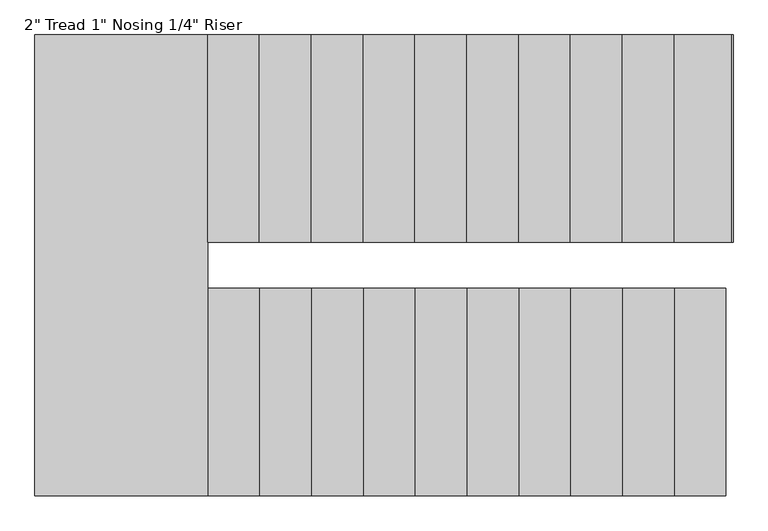
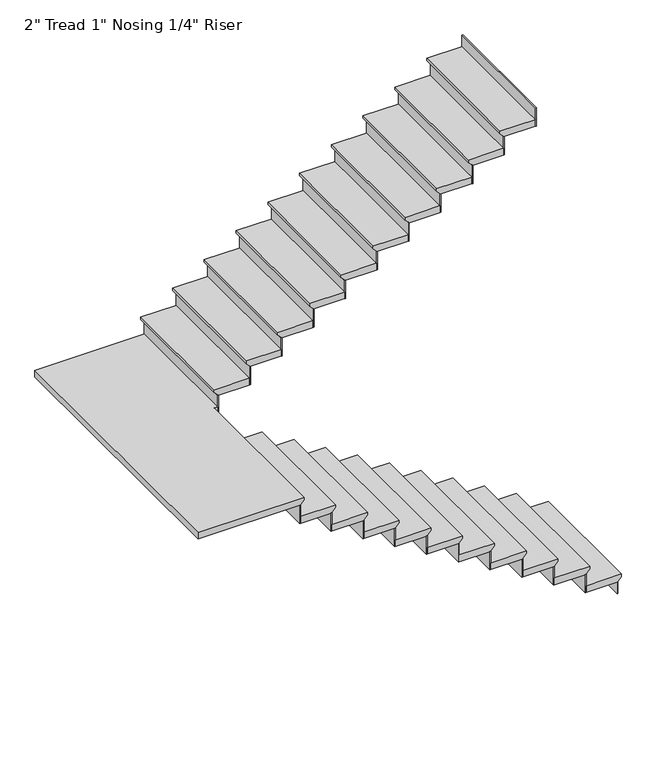
"""IFC4 building model written with IfcOpenShell, lengths in millimetres: stair flight geometry."""

from ifc_helpers import new_model, si_unit, origin, place, context, project, spatial, faceted_brep, source, transform, mapped, element, save


def stair_flight_f9c943de(model_context):
    return source(origin(), model_context, "Body", "Brep", [
        faceted_brep([(-2080.8410855, 332.1803617, 9720.6954545), (-2080.8410855, 332.1803617, 9739.7454545), (-2080.8410855, -582.2196383, 9739.7454545), (-2080.8410855, -582.2196383, 9720.6954545), (-2106.2410855, 332.1803617, 9695.2954545), (-2106.2410855, -582.2196383, 9695.2954545), (-2334.8410855, 332.1803617, 9739.7454545), (-2334.8410855, -582.2196383, 9739.7454545), (-2106.2410855, -582.2196383, 9688.9454545), (-2334.8410855, -582.2196383, 9688.9454545), (-2334.8410855, 332.1803617, 9688.9454545), (-2106.2410855, 332.1803617, 9688.9454545)], [[[0, 1, 2, 3]], [[4, 0, 3, 5]], [[2, 1, 6, 7]], [[8, 9, 10, 11]], [[2, 7, 9, 8, 5, 3]], [[8, 11, 4, 5]], [[6, 1, 0, 4, 11, 10]], [[7, 6, 10, 9]]]),
        faceted_brep([(-2106.2410855, 332.1803617, 9688.9454545), (-2106.2410855, 332.1803617, 9601.2), (-2112.5910855, 332.1803617, 9601.2), (-2112.5910855, 332.1803617, 9688.9454545), (-2106.2410855, -582.2196383, 9688.9454545), (-2112.5910855, -582.2196383, 9688.9454545), (-2112.5910855, -582.2196383, 9601.2), (-2106.2410855, -582.2196383, 9601.2)], [[[0, 1, 2, 3]], [[4, 5, 6, 7]], [[1, 0, 4, 7]], [[2, 1, 7, 6]], [[3, 2, 6, 5]], [[0, 3, 5, 4]]]),
        faceted_brep([(-2334.8410855, 332.1803617, 9827.4909091), (-2334.8410855, 332.1803617, 9688.9454545), (-2341.1910855, 332.1803617, 9688.9454545), (-2341.1910855, 332.1803617, 9827.4909091), (-2334.8410855, -582.2196383, 9827.4909091), (-2341.1910855, -582.2196383, 9827.4909091), (-2341.1910855, -582.2196383, 9688.9454545), (-2334.8410855, -582.2196383, 9688.9454545)], [[[0, 1, 2, 3]], [[4, 5, 6, 7]], [[1, 0, 4, 7]], [[2, 1, 7, 6]], [[3, 2, 6, 5]], [[0, 3, 5, 4]]]),
        faceted_brep([(-2309.4410855, -582.2196383, 9878.2909091), (-2309.4410855, 332.1803617, 9878.2909091), (-2563.4410855, 332.1803617, 9878.2909091), (-2563.4410855, -582.2196383, 9878.2909091), (-2334.8410855, -582.2196383, 9827.4909091), (-2563.4410855, -582.2196383, 9827.4909091), (-2563.4410855, 332.1803617, 9827.4909091), (-2334.8410855, 332.1803617, 9827.4909091), (-2334.8410855, -582.2196383, 9833.8409091), (-2309.4410855, -582.2196383, 9859.2409091), (-2334.8410855, 332.1803617, 9833.8409091), (-2309.4410855, 332.1803617, 9859.2409091)], [[[0, 1, 2, 3]], [[4, 5, 6, 7]], [[0, 3, 5, 4, 8, 9]], [[4, 7, 10, 8]], [[2, 1, 11, 10, 7, 6]], [[3, 2, 6, 5]], [[11, 1, 0, 9]], [[10, 11, 9, 8]]]),
        faceted_brep([(-2563.4410855, 332.1803617, 9966.0363636), (-2563.4410855, 332.1803617, 9827.4909091), (-2569.7910855, 332.1803617, 9827.4909091), (-2569.7910855, 332.1803617, 9966.0363636), (-2563.4410855, -582.2196383, 9966.0363636), (-2569.7910855, -582.2196383, 9966.0363636), (-2569.7910855, -582.2196383, 9827.4909091), (-2563.4410855, -582.2196383, 9827.4909091)], [[[0, 1, 2, 3]], [[4, 5, 6, 7]], [[1, 0, 4, 7]], [[2, 1, 7, 6]], [[3, 2, 6, 5]], [[0, 3, 5, 4]]]),
        faceted_brep([(-2538.0410855, -582.2196383, 10016.8363636), (-2538.0410855, 332.1803617, 10016.8363636), (-2792.0410855, 332.1803617, 10016.8363636), (-2792.0410855, -582.2196383, 10016.8363636), (-2563.4410855, -582.2196383, 9966.0363636), (-2792.0410855, -582.2196383, 9966.0363636), (-2792.0410855, 332.1803617, 9966.0363636), (-2563.4410855, 332.1803617, 9966.0363636), (-2563.4410855, -582.2196383, 9972.3863636), (-2538.0410855, -582.2196383, 9997.7863636), (-2563.4410855, 332.1803617, 9972.3863636), (-2538.0410855, 332.1803617, 9997.7863636)], [[[0, 1, 2, 3]], [[4, 5, 6, 7]], [[0, 3, 5, 4, 8, 9]], [[4, 7, 10, 8]], [[2, 1, 11, 10, 7, 6]], [[3, 2, 6, 5]], [[11, 1, 0, 9]], [[10, 11, 9, 8]]]),
        faceted_brep([(-2792.0410855, 332.1803617, 10104.5818182), (-2792.0410855, 332.1803617, 9966.0363636), (-2798.3910855, 332.1803617, 9966.0363636), (-2798.3910855, 332.1803617, 10104.5818182), (-2792.0410855, -582.2196383, 10104.5818182), (-2798.3910855, -582.2196383, 10104.5818182), (-2798.3910855, -582.2196383, 9966.0363636), (-2792.0410855, -582.2196383, 9966.0363636)], [[[0, 1, 2, 3]], [[4, 5, 6, 7]], [[1, 0, 4, 7]], [[2, 1, 7, 6]], [[3, 2, 6, 5]], [[0, 3, 5, 4]]]),
        faceted_brep([(-2766.6410855, -582.2196383, 10155.3818182), (-2766.6410855, 332.1803617, 10155.3818182), (-3020.6410855, 332.1803617, 10155.3818182), (-3020.6410855, -582.2196383, 10155.3818182), (-2792.0410855, -582.2196383, 10104.5818182), (-3020.6410855, -582.2196383, 10104.5818182), (-3020.6410855, 332.1803617, 10104.5818182), (-2792.0410855, 332.1803617, 10104.5818182), (-2792.0410855, -582.2196383, 10110.9318182), (-2766.6410855, -582.2196383, 10136.3318182), (-2792.0410855, 332.1803617, 10110.9318182), (-2766.6410855, 332.1803617, 10136.3318182)], [[[0, 1, 2, 3]], [[4, 5, 6, 7]], [[0, 3, 5, 4, 8, 9]], [[4, 7, 10, 8]], [[2, 1, 11, 10, 7, 6]], [[3, 2, 6, 5]], [[11, 1, 0, 9]], [[10, 11, 9, 8]]]),
        faceted_brep([(-3020.6410855, 332.1803617, 10243.1272727), (-3020.6410855, 332.1803617, 10104.5818182), (-3026.9910855, 332.1803617, 10104.5818182), (-3026.9910855, 332.1803617, 10243.1272727), (-3020.6410855, -582.2196383, 10243.1272727), (-3026.9910855, -582.2196383, 10243.1272727), (-3026.9910855, -582.2196383, 10104.5818182), (-3020.6410855, -582.2196383, 10104.5818182)], [[[0, 1, 2, 3]], [[4, 5, 6, 7]], [[1, 0, 4, 7]], [[2, 1, 7, 6]], [[3, 2, 6, 5]], [[0, 3, 5, 4]]]),
        faceted_brep([(-2995.2410855, -582.2196383, 10293.9272727), (-2995.2410855, 332.1803617, 10293.9272727), (-3249.2410855, 332.1803617, 10293.9272727), (-3249.2410855, -582.2196383, 10293.9272727), (-3020.6410855, -582.2196383, 10243.1272727), (-3249.2410855, -582.2196383, 10243.1272727), (-3249.2410855, 332.1803617, 10243.1272727), (-3020.6410855, 332.1803617, 10243.1272727), (-3020.6410855, -582.2196383, 10249.4772727), (-2995.2410855, -582.2196383, 10274.8772727), (-3020.6410855, 332.1803617, 10249.4772727), (-2995.2410855, 332.1803617, 10274.8772727)], [[[0, 1, 2, 3]], [[4, 5, 6, 7]], [[0, 3, 5, 4, 8, 9]], [[4, 7, 10, 8]], [[2, 1, 11, 10, 7, 6]], [[3, 2, 6, 5]], [[11, 1, 0, 9]], [[10, 11, 9, 8]]]),
        faceted_brep([(-3249.2410855, 332.1803617, 10381.6727273), (-3249.2410855, 332.1803617, 10243.1272727), (-3255.5910855, 332.1803617, 10243.1272727), (-3255.5910855, 332.1803617, 10381.6727273), (-3249.2410855, -582.2196383, 10381.6727273), (-3255.5910855, -582.2196383, 10381.6727273), (-3255.5910855, -582.2196383, 10243.1272727), (-3249.2410855, -582.2196383, 10243.1272727)], [[[0, 1, 2, 3]], [[4, 5, 6, 7]], [[1, 0, 4, 7]], [[2, 1, 7, 6]], [[3, 2, 6, 5]], [[0, 3, 5, 4]]]),
        faceted_brep([(-3223.8410855, -582.2196383, 10432.4727273), (-3223.8410855, 332.1803617, 10432.4727273), (-3477.8410855, 332.1803617, 10432.4727273), (-3477.8410855, -582.2196383, 10432.4727273), (-3249.2410855, -582.2196383, 10381.6727273), (-3477.8410855, -582.2196383, 10381.6727273), (-3477.8410855, 332.1803617, 10381.6727273), (-3249.2410855, 332.1803617, 10381.6727273), (-3249.2410855, -582.2196383, 10388.0227273), (-3223.8410855, -582.2196383, 10413.4227273), (-3249.2410855, 332.1803617, 10388.0227273), (-3223.8410855, 332.1803617, 10413.4227273)], [[[0, 1, 2, 3]], [[4, 5, 6, 7]], [[0, 3, 5, 4, 8, 9]], [[4, 7, 10, 8]], [[2, 1, 11, 10, 7, 6]], [[3, 2, 6, 5]], [[11, 1, 0, 9]], [[10, 11, 9, 8]]]),
        faceted_brep([(-3477.8410855, 332.1803617, 10520.2181818), (-3477.8410855, 332.1803617, 10381.6727273), (-3484.1910855, 332.1803617, 10381.6727273), (-3484.1910855, 332.1803617, 10520.2181818), (-3477.8410855, -582.2196383, 10520.2181818), (-3484.1910855, -582.2196383, 10520.2181818), (-3484.1910855, -582.2196383, 10381.6727273), (-3477.8410855, -582.2196383, 10381.6727273)], [[[0, 1, 2, 3]], [[4, 5, 6, 7]], [[1, 0, 4, 7]], [[2, 1, 7, 6]], [[3, 2, 6, 5]], [[0, 3, 5, 4]]]),
        faceted_brep([(-3452.4410855, -582.2196383, 10571.0181818), (-3452.4410855, 332.1803617, 10571.0181818), (-3706.4410855, 332.1803617, 10571.0181818), (-3706.4410855, -582.2196383, 10571.0181818), (-3477.8410855, -582.2196383, 10520.2181818), (-3706.4410855, -582.2196383, 10520.2181818), (-3706.4410855, 332.1803617, 10520.2181818), (-3477.8410855, 332.1803617, 10520.2181818), (-3477.8410855, -582.2196383, 10526.5681818), (-3452.4410855, -582.2196383, 10551.9681818), (-3477.8410855, 332.1803617, 10526.5681818), (-3452.4410855, 332.1803617, 10551.9681818)], [[[0, 1, 2, 3]], [[4, 5, 6, 7]], [[0, 3, 5, 4, 8, 9]], [[4, 7, 10, 8]], [[2, 1, 11, 10, 7, 6]], [[3, 2, 6, 5]], [[11, 1, 0, 9]], [[10, 11, 9, 8]]]),
        faceted_brep([(-3706.4410855, 332.1803617, 10658.7636364), (-3706.4410855, 332.1803617, 10520.2181818), (-3712.7910855, 332.1803617, 10520.2181818), (-3712.7910855, 332.1803617, 10658.7636364), (-3706.4410855, -582.2196383, 10658.7636364), (-3712.7910855, -582.2196383, 10658.7636364), (-3712.7910855, -582.2196383, 10520.2181818), (-3706.4410855, -582.2196383, 10520.2181818)], [[[0, 1, 2, 3]], [[4, 5, 6, 7]], [[1, 0, 4, 7]], [[2, 1, 7, 6]], [[3, 2, 6, 5]], [[0, 3, 5, 4]]]),
        faceted_brep([(-3681.0410855, -582.2196383, 10709.5636364), (-3681.0410855, 332.1803617, 10709.5636364), (-3935.0410855, 332.1803617, 10709.5636364), (-3935.0410855, -582.2196383, 10709.5636364), (-3706.4410855, -582.2196383, 10658.7636364), (-3935.0410855, -582.2196383, 10658.7636364), (-3935.0410855, 332.1803617, 10658.7636364), (-3706.4410855, 332.1803617, 10658.7636364), (-3706.4410855, -582.2196383, 10665.1136364), (-3681.0410855, -582.2196383, 10690.5136364), (-3706.4410855, 332.1803617, 10665.1136364), (-3681.0410855, 332.1803617, 10690.5136364)], [[[0, 1, 2, 3]], [[4, 5, 6, 7]], [[0, 3, 5, 4, 8, 9]], [[4, 7, 10, 8]], [[2, 1, 11, 10, 7, 6]], [[3, 2, 6, 5]], [[11, 1, 0, 9]], [[10, 11, 9, 8]]]),
        faceted_brep([(-3935.0410855, 332.1803617, 10797.3090909), (-3935.0410855, 332.1803617, 10658.7636364), (-3941.3910855, 332.1803617, 10658.7636364), (-3941.3910855, 332.1803617, 10797.3090909), (-3935.0410855, -582.2196383, 10797.3090909), (-3941.3910855, -582.2196383, 10797.3090909), (-3941.3910855, -582.2196383, 10658.7636364), (-3935.0410855, -582.2196383, 10658.7636364)], [[[0, 1, 2, 3]], [[4, 5, 6, 7]], [[1, 0, 4, 7]], [[2, 1, 7, 6]], [[3, 2, 6, 5]], [[0, 3, 5, 4]]]),
        faceted_brep([(-3909.6410855, -582.2196383, 10848.1090909), (-3909.6410855, 332.1803617, 10848.1090909), (-4163.6410855, 332.1803617, 10848.1090909), (-4163.6410855, -582.2196383, 10848.1090909), (-3935.0410855, -582.2196383, 10797.3090909), (-4163.6410855, -582.2196383, 10797.3090909), (-4163.6410855, 332.1803617, 10797.3090909), (-3935.0410855, 332.1803617, 10797.3090909), (-3935.0410855, -582.2196383, 10803.6590909), (-3909.6410855, -582.2196383, 10829.0590909), (-3935.0410855, 332.1803617, 10803.6590909), (-3909.6410855, 332.1803617, 10829.0590909)], [[[0, 1, 2, 3]], [[4, 5, 6, 7]], [[0, 3, 5, 4, 8, 9]], [[4, 7, 10, 8]], [[2, 1, 11, 10, 7, 6]], [[3, 2, 6, 5]], [[11, 1, 0, 9]], [[10, 11, 9, 8]]]),
        faceted_brep([(-4163.6410855, 332.1803617, 10935.8545455), (-4163.6410855, 332.1803617, 10797.3090909), (-4169.9910855, 332.1803617, 10797.3090909), (-4169.9910855, 332.1803617, 10935.8545455), (-4163.6410855, -582.2196383, 10935.8545455), (-4169.9910855, -582.2196383, 10935.8545455), (-4169.9910855, -582.2196383, 10797.3090909), (-4163.6410855, -582.2196383, 10797.3090909)], [[[0, 1, 2, 3]], [[4, 5, 6, 7]], [[1, 0, 4, 7]], [[2, 1, 7, 6]], [[3, 2, 6, 5]], [[0, 3, 5, 4]]]),
        faceted_brep([(-4138.2410855, -582.2196383, 10986.6545455), (-4138.2410855, 332.1803617, 10986.6545455), (-4392.2410855, 332.1803617, 10986.6545455), (-4392.2410855, -582.2196383, 10986.6545455), (-4163.6410855, -582.2196383, 10935.8545455), (-4392.2410855, -582.2196383, 10935.8545455), (-4392.2410855, 332.1803617, 10935.8545455), (-4163.6410855, 332.1803617, 10935.8545455), (-4163.6410855, -582.2196383, 10942.2045455), (-4138.2410855, -582.2196383, 10967.6045455), (-4163.6410855, 332.1803617, 10942.2045455), (-4138.2410855, 332.1803617, 10967.6045455)], [[[0, 1, 2, 3]], [[4, 5, 6, 7]], [[0, 3, 5, 4, 8, 9]], [[4, 7, 10, 8]], [[2, 1, 11, 10, 7, 6]], [[3, 2, 6, 5]], [[11, 1, 0, 9]], [[10, 11, 9, 8]]]),
        faceted_brep([(-4392.2410855, 332.1803617, 11074.4), (-4392.2410855, 332.1803617, 10935.8545455), (-4398.5910855, 332.1803617, 10935.8545455), (-4398.5910855, 332.1803617, 11074.4), (-4392.2410855, -582.2196383, 11074.4), (-4398.5910855, -582.2196383, 11074.4), (-4398.5910855, -582.2196383, 10935.8545455), (-4392.2410855, -582.2196383, 10935.8545455)], [[[0, 1, 2, 3]], [[4, 5, 6, 7]], [[1, 0, 4, 7]], [[2, 1, 7, 6]], [[3, 2, 6, 5]], [[0, 3, 5, 4]]]),
        faceted_brep([(-4341.4410855, 1449.7803617, 11125.2), (-5128.8410855, 1449.7803617, 11125.2), (-5128.8410855, -582.2196383, 11125.2), (-4366.8410855, -582.2196383, 11125.2), (-4366.8410855, 535.3803617, 11125.2), (-4341.4410855, 535.3803617, 11125.2), (-5128.8410855, 1449.7803617, 11074.4), (-4341.4410855, 1449.7803617, 11074.4), (-4341.4410855, 535.3803617, 11074.4), (-4366.8410855, 535.3803617, 11074.4), (-4366.8410855, 332.1803617, 11074.4), (-4392.2410855, 332.1803617, 11074.4), (-4392.2410855, -582.2196383, 11074.4), (-5128.8410855, -582.2196383, 11074.4), (-4392.2410855, -582.2196383, 11080.75), (-4366.8410855, -582.2196383, 11106.15), (-4392.2410855, 332.1803617, 11080.75), (-4366.8410855, 332.1803617, 11106.15)], [[[0, 1, 2, 3, 4, 5]], [[6, 7, 8, 9, 10, 11, 12, 13]], [[1, 0, 7, 6]], [[2, 1, 6, 13]], [[3, 2, 13, 12, 14, 15]], [[12, 11, 16, 14]], [[11, 10, 17, 16]], [[4, 3, 15, 17, 10, 9]], [[5, 4, 9, 8]], [[0, 5, 8, 7]], [[15, 14, 16, 17]]]),
        faceted_brep([(-4341.4410855, 535.3803617, 11212.9454545), (-4341.4410855, 535.3803617, 11074.4), (-4335.0910855, 535.3803617, 11074.4), (-4335.0910855, 535.3803617, 11212.9454545), (-4341.4410855, 1449.7803617, 11212.9454545), (-4335.0910855, 1449.7803617, 11212.9454545), (-4335.0910855, 1449.7803617, 11074.4), (-4341.4410855, 1449.7803617, 11074.4)], [[[0, 1, 2, 3]], [[4, 5, 6, 7]], [[1, 0, 4, 7]], [[2, 1, 7, 6]], [[3, 2, 6, 5]], [[0, 3, 5, 4]]]),
        faceted_brep([(-4366.8410855, 1449.7803617, 11263.7454545), (-4366.8410855, 535.3803617, 11263.7454545), (-4112.8410855, 535.3803617, 11263.7454545), (-4112.8410855, 1449.7803617, 11263.7454545), (-4341.4410855, 1449.7803617, 11212.9454545), (-4112.8410855, 1449.7803617, 11212.9454545), (-4112.8410855, 535.3803617, 11212.9454545), (-4341.4410855, 535.3803617, 11212.9454545), (-4341.4410855, 1449.7803617, 11219.2954545), (-4366.8410855, 1449.7803617, 11244.6954545), (-4341.4410855, 535.3803617, 11219.2954545), (-4366.8410855, 535.3803617, 11244.6954545)], [[[0, 1, 2, 3]], [[4, 5, 6, 7]], [[0, 3, 5, 4, 8, 9]], [[4, 7, 10, 8]], [[2, 1, 11, 10, 7, 6]], [[3, 2, 6, 5]], [[11, 1, 0, 9]], [[10, 11, 9, 8]]]),
        faceted_brep([(-4112.8410855, 535.3803617, 11351.4909091), (-4112.8410855, 535.3803617, 11212.9454545), (-4106.4910855, 535.3803617, 11212.9454545), (-4106.4910855, 535.3803617, 11351.4909091), (-4112.8410855, 1449.7803617, 11351.4909091), (-4106.4910855, 1449.7803617, 11351.4909091), (-4106.4910855, 1449.7803617, 11212.9454545), (-4112.8410855, 1449.7803617, 11212.9454545)], [[[0, 1, 2, 3]], [[4, 5, 6, 7]], [[1, 0, 4, 7]], [[2, 1, 7, 6]], [[3, 2, 6, 5]], [[0, 3, 5, 4]]]),
        faceted_brep([(-4138.2410855, 1449.7803617, 11402.2909091), (-4138.2410855, 535.3803617, 11402.2909091), (-3884.2410855, 535.3803617, 11402.2909091), (-3884.2410855, 1449.7803617, 11402.2909091), (-4112.8410855, 1449.7803617, 11351.4909091), (-3884.2410855, 1449.7803617, 11351.4909091), (-3884.2410855, 535.3803617, 11351.4909091), (-4112.8410855, 535.3803617, 11351.4909091), (-4112.8410855, 1449.7803617, 11357.8409091), (-4138.2410855, 1449.7803617, 11383.2409091), (-4112.8410855, 535.3803617, 11357.8409091), (-4138.2410855, 535.3803617, 11383.2409091)], [[[0, 1, 2, 3]], [[4, 5, 6, 7]], [[0, 3, 5, 4, 8, 9]], [[4, 7, 10, 8]], [[2, 1, 11, 10, 7, 6]], [[3, 2, 6, 5]], [[11, 1, 0, 9]], [[10, 11, 9, 8]]]),
        faceted_brep([(-3884.2410855, 535.3803617, 11490.0363636), (-3884.2410855, 535.3803617, 11351.4909091), (-3877.8910855, 535.3803617, 11351.4909091), (-3877.8910855, 535.3803617, 11490.0363636), (-3884.2410855, 1449.7803617, 11490.0363636), (-3877.8910855, 1449.7803617, 11490.0363636), (-3877.8910855, 1449.7803617, 11351.4909091), (-3884.2410855, 1449.7803617, 11351.4909091)], [[[0, 1, 2, 3]], [[4, 5, 6, 7]], [[1, 0, 4, 7]], [[2, 1, 7, 6]], [[3, 2, 6, 5]], [[0, 3, 5, 4]]]),
        faceted_brep([(-3909.6410855, 1449.7803617, 11540.8363636), (-3909.6410855, 535.3803617, 11540.8363636), (-3655.6410855, 535.3803617, 11540.8363636), (-3655.6410855, 1449.7803617, 11540.8363636), (-3884.2410855, 1449.7803617, 11490.0363636), (-3655.6410855, 1449.7803617, 11490.0363636), (-3655.6410855, 535.3803617, 11490.0363636), (-3884.2410855, 535.3803617, 11490.0363636), (-3884.2410855, 1449.7803617, 11496.3863636), (-3909.6410855, 1449.7803617, 11521.7863636), (-3884.2410855, 535.3803617, 11496.3863636), (-3909.6410855, 535.3803617, 11521.7863636)], [[[0, 1, 2, 3]], [[4, 5, 6, 7]], [[0, 3, 5, 4, 8, 9]], [[4, 7, 10, 8]], [[2, 1, 11, 10, 7, 6]], [[3, 2, 6, 5]], [[11, 1, 0, 9]], [[10, 11, 9, 8]]]),
        faceted_brep([(-3655.6410855, 535.3803617, 11628.5818182), (-3655.6410855, 535.3803617, 11490.0363636), (-3649.2910855, 535.3803617, 11490.0363636), (-3649.2910855, 535.3803617, 11628.5818182), (-3655.6410855, 1449.7803617, 11628.5818182), (-3649.2910855, 1449.7803617, 11628.5818182), (-3649.2910855, 1449.7803617, 11490.0363636), (-3655.6410855, 1449.7803617, 11490.0363636)], [[[0, 1, 2, 3]], [[4, 5, 6, 7]], [[1, 0, 4, 7]], [[2, 1, 7, 6]], [[3, 2, 6, 5]], [[0, 3, 5, 4]]]),
        faceted_brep([(-3681.0410855, 1449.7803617, 11679.3818182), (-3681.0410855, 535.3803617, 11679.3818182), (-3427.0410855, 535.3803617, 11679.3818182), (-3427.0410855, 1449.7803617, 11679.3818182), (-3655.6410855, 1449.7803617, 11628.5818182), (-3427.0410855, 1449.7803617, 11628.5818182), (-3427.0410855, 535.3803617, 11628.5818182), (-3655.6410855, 535.3803617, 11628.5818182), (-3655.6410855, 1449.7803617, 11634.9318182), (-3681.0410855, 1449.7803617, 11660.3318182), (-3655.6410855, 535.3803617, 11634.9318182), (-3681.0410855, 535.3803617, 11660.3318182)], [[[0, 1, 2, 3]], [[4, 5, 6, 7]], [[0, 3, 5, 4, 8, 9]], [[4, 7, 10, 8]], [[2, 1, 11, 10, 7, 6]], [[3, 2, 6, 5]], [[11, 1, 0, 9]], [[10, 11, 9, 8]]]),
        faceted_brep([(-3427.0410855, 535.3803617, 11767.1272727), (-3427.0410855, 535.3803617, 11628.5818182), (-3420.6910855, 535.3803617, 11628.5818182), (-3420.6910855, 535.3803617, 11767.1272727), (-3427.0410855, 1449.7803617, 11767.1272727), (-3420.6910855, 1449.7803617, 11767.1272727), (-3420.6910855, 1449.7803617, 11628.5818182), (-3427.0410855, 1449.7803617, 11628.5818182)], [[[0, 1, 2, 3]], [[4, 5, 6, 7]], [[1, 0, 4, 7]], [[2, 1, 7, 6]], [[3, 2, 6, 5]], [[0, 3, 5, 4]]]),
        faceted_brep([(-3452.4410855, 1449.7803617, 11817.9272727), (-3452.4410855, 535.3803617, 11817.9272727), (-3198.4410855, 535.3803617, 11817.9272727), (-3198.4410855, 1449.7803617, 11817.9272727), (-3427.0410855, 1449.7803617, 11767.1272727), (-3198.4410855, 1449.7803617, 11767.1272727), (-3198.4410855, 535.3803617, 11767.1272727), (-3427.0410855, 535.3803617, 11767.1272727), (-3427.0410855, 1449.7803617, 11773.4772727), (-3452.4410855, 1449.7803617, 11798.8772727), (-3427.0410855, 535.3803617, 11773.4772727), (-3452.4410855, 535.3803617, 11798.8772727)], [[[0, 1, 2, 3]], [[4, 5, 6, 7]], [[0, 3, 5, 4, 8, 9]], [[4, 7, 10, 8]], [[2, 1, 11, 10, 7, 6]], [[3, 2, 6, 5]], [[11, 1, 0, 9]], [[10, 11, 9, 8]]]),
        faceted_brep([(-3198.4410855, 535.3803617, 11905.6727273), (-3198.4410855, 535.3803617, 11767.1272727), (-3192.0910855, 535.3803617, 11767.1272727), (-3192.0910855, 535.3803617, 11905.6727273), (-3198.4410855, 1449.7803617, 11905.6727273), (-3192.0910855, 1449.7803617, 11905.6727273), (-3192.0910855, 1449.7803617, 11767.1272727), (-3198.4410855, 1449.7803617, 11767.1272727)], [[[0, 1, 2, 3]], [[4, 5, 6, 7]], [[1, 0, 4, 7]], [[2, 1, 7, 6]], [[3, 2, 6, 5]], [[0, 3, 5, 4]]]),
        faceted_brep([(-3223.8410855, 1449.7803617, 11956.4727273), (-3223.8410855, 535.3803617, 11956.4727273), (-2969.8410855, 535.3803617, 11956.4727273), (-2969.8410855, 1449.7803617, 11956.4727273), (-3198.4410855, 1449.7803617, 11905.6727273), (-2969.8410855, 1449.7803617, 11905.6727273), (-2969.8410855, 535.3803617, 11905.6727273), (-3198.4410855, 535.3803617, 11905.6727273), (-3198.4410855, 1449.7803617, 11912.0227273), (-3223.8410855, 1449.7803617, 11937.4227273), (-3198.4410855, 535.3803617, 11912.0227273), (-3223.8410855, 535.3803617, 11937.4227273)], [[[0, 1, 2, 3]], [[4, 5, 6, 7]], [[0, 3, 5, 4, 8, 9]], [[4, 7, 10, 8]], [[2, 1, 11, 10, 7, 6]], [[3, 2, 6, 5]], [[11, 1, 0, 9]], [[10, 11, 9, 8]]]),
        faceted_brep([(-2969.8410855, 535.3803617, 12044.2181818), (-2969.8410855, 535.3803617, 11905.6727273), (-2963.4910855, 535.3803617, 11905.6727273), (-2963.4910855, 535.3803617, 12044.2181818), (-2969.8410855, 1449.7803617, 12044.2181818), (-2963.4910855, 1449.7803617, 12044.2181818), (-2963.4910855, 1449.7803617, 11905.6727273), (-2969.8410855, 1449.7803617, 11905.6727273)], [[[0, 1, 2, 3]], [[4, 5, 6, 7]], [[1, 0, 4, 7]], [[2, 1, 7, 6]], [[3, 2, 6, 5]], [[0, 3, 5, 4]]]),
        faceted_brep([(-2995.2410855, 1449.7803617, 12095.0181818), (-2995.2410855, 535.3803617, 12095.0181818), (-2741.2410855, 535.3803617, 12095.0181818), (-2741.2410855, 1449.7803617, 12095.0181818), (-2969.8410855, 1449.7803617, 12044.2181818), (-2741.2410855, 1449.7803617, 12044.2181818), (-2741.2410855, 535.3803617, 12044.2181818), (-2969.8410855, 535.3803617, 12044.2181818), (-2969.8410855, 1449.7803617, 12050.5681818), (-2995.2410855, 1449.7803617, 12075.9681818), (-2969.8410855, 535.3803617, 12050.5681818), (-2995.2410855, 535.3803617, 12075.9681818)], [[[0, 1, 2, 3]], [[4, 5, 6, 7]], [[0, 3, 5, 4, 8, 9]], [[4, 7, 10, 8]], [[2, 1, 11, 10, 7, 6]], [[3, 2, 6, 5]], [[11, 1, 0, 9]], [[10, 11, 9, 8]]]),
        faceted_brep([(-2741.2410855, 535.3803617, 12182.7636364), (-2741.2410855, 535.3803617, 12044.2181818), (-2734.8910855, 535.3803617, 12044.2181818), (-2734.8910855, 535.3803617, 12182.7636364), (-2741.2410855, 1449.7803617, 12182.7636364), (-2734.8910855, 1449.7803617, 12182.7636364), (-2734.8910855, 1449.7803617, 12044.2181818), (-2741.2410855, 1449.7803617, 12044.2181818)], [[[0, 1, 2, 3]], [[4, 5, 6, 7]], [[1, 0, 4, 7]], [[2, 1, 7, 6]], [[3, 2, 6, 5]], [[0, 3, 5, 4]]]),
        faceted_brep([(-2766.6410855, 1449.7803617, 12233.5636364), (-2766.6410855, 535.3803617, 12233.5636364), (-2512.6410855, 535.3803617, 12233.5636364), (-2512.6410855, 1449.7803617, 12233.5636364), (-2741.2410855, 1449.7803617, 12182.7636364), (-2512.6410855, 1449.7803617, 12182.7636364), (-2512.6410855, 535.3803617, 12182.7636364), (-2741.2410855, 535.3803617, 12182.7636364), (-2741.2410855, 1449.7803617, 12189.1136364), (-2766.6410855, 1449.7803617, 12214.5136364), (-2741.2410855, 535.3803617, 12189.1136364), (-2766.6410855, 535.3803617, 12214.5136364)], [[[0, 1, 2, 3]], [[4, 5, 6, 7]], [[0, 3, 5, 4, 8, 9]], [[4, 7, 10, 8]], [[2, 1, 11, 10, 7, 6]], [[3, 2, 6, 5]], [[11, 1, 0, 9]], [[10, 11, 9, 8]]]),
        faceted_brep([(-2512.6410855, 535.3803617, 12321.3090909), (-2512.6410855, 535.3803617, 12182.7636364), (-2506.2910855, 535.3803617, 12182.7636364), (-2506.2910855, 535.3803617, 12321.3090909), (-2512.6410855, 1449.7803617, 12321.3090909), (-2506.2910855, 1449.7803617, 12321.3090909), (-2506.2910855, 1449.7803617, 12182.7636364), (-2512.6410855, 1449.7803617, 12182.7636364)], [[[0, 1, 2, 3]], [[4, 5, 6, 7]], [[1, 0, 4, 7]], [[2, 1, 7, 6]], [[3, 2, 6, 5]], [[0, 3, 5, 4]]]),
        faceted_brep([(-2538.0410855, 1449.7803617, 12372.1090909), (-2538.0410855, 535.3803617, 12372.1090909), (-2284.0410855, 535.3803617, 12372.1090909), (-2284.0410855, 1449.7803617, 12372.1090909), (-2512.6410855, 1449.7803617, 12321.3090909), (-2284.0410855, 1449.7803617, 12321.3090909), (-2284.0410855, 535.3803617, 12321.3090909), (-2512.6410855, 535.3803617, 12321.3090909), (-2512.6410855, 1449.7803617, 12327.6590909), (-2538.0410855, 1449.7803617, 12353.0590909), (-2512.6410855, 535.3803617, 12327.6590909), (-2538.0410855, 535.3803617, 12353.0590909)], [[[0, 1, 2, 3]], [[4, 5, 6, 7]], [[0, 3, 5, 4, 8, 9]], [[4, 7, 10, 8]], [[2, 1, 11, 10, 7, 6]], [[3, 2, 6, 5]], [[11, 1, 0, 9]], [[10, 11, 9, 8]]]),
        faceted_brep([(-2284.0410855, 535.3803617, 12459.8545455), (-2284.0410855, 535.3803617, 12321.3090909), (-2277.6910855, 535.3803617, 12321.3090909), (-2277.6910855, 535.3803617, 12459.8545455), (-2284.0410855, 1449.7803617, 12459.8545455), (-2277.6910855, 1449.7803617, 12459.8545455), (-2277.6910855, 1449.7803617, 12321.3090909), (-2284.0410855, 1449.7803617, 12321.3090909)], [[[0, 1, 2, 3]], [[4, 5, 6, 7]], [[1, 0, 4, 7]], [[2, 1, 7, 6]], [[3, 2, 6, 5]], [[0, 3, 5, 4]]]),
        faceted_brep([(-2055.4410855, 535.3803617, 12598.4), (-2055.4410855, 535.3803617, 12459.8545455), (-2049.0910855, 535.3803617, 12459.8545455), (-2049.0910855, 535.3803617, 12598.4), (-2055.4410855, 1449.7803617, 12598.4), (-2049.0910855, 1449.7803617, 12598.4), (-2049.0910855, 1449.7803617, 12459.8545455), (-2055.4410855, 1449.7803617, 12459.8545455)], [[[0, 1, 2, 3]], [[4, 5, 6, 7]], [[1, 0, 4, 7]], [[2, 1, 7, 6]], [[3, 2, 6, 5]], [[0, 3, 5, 4]]]),
        faceted_brep([(-2309.4410855, 1449.7803617, 12510.6545455), (-2309.4410855, 535.3803617, 12510.6545455), (-2055.4410855, 535.3803617, 12510.6545455), (-2055.4410855, 1449.7803617, 12510.6545455), (-2284.0410855, 1449.7803617, 12459.8545455), (-2055.4410855, 1449.7803617, 12459.8545455), (-2055.4410855, 535.3803617, 12459.8545455), (-2284.0410855, 535.3803617, 12459.8545455), (-2284.0410855, 1449.7803617, 12466.2045455), (-2309.4410855, 1449.7803617, 12491.6045455), (-2284.0410855, 535.3803617, 12466.2045455), (-2309.4410855, 535.3803617, 12491.6045455)], [[[0, 1, 2, 3]], [[4, 5, 6, 7]], [[0, 3, 5, 4, 8, 9]], [[4, 7, 10, 8]], [[2, 1, 11, 10, 7, 6]], [[3, 2, 6, 5]], [[11, 1, 0, 9]], [[10, 11, 9, 8]]]),
    ])


if __name__ == "__main__":
    model = new_model("IFC4")
    model_context = context("Model", 3, world=origin())
    ifc_project = project(units=[si_unit("LENGTHUNIT", "METRE", prefix="MILLI")], contexts=[model_context])
    site = spatial("IfcSite", under=ifc_project)
    building = spatial("IfcBuilding", under=site)
    placement = place(None, origin())
    stair_flight_shape = stair_flight_f9c943de(model_context)
    element("IfcStairFlight", 1, ObjectType="2\" Tread 1\" Nosing 1/4\" Riser", at=placement, inside=building, context=model_context, shape_type="MappedRepresentation", body=[
        mapped(stair_flight_shape, transform((0.0, 0.0, 0.0), x_axis=(1.0, 0.0, 0.0), y_axis=(0.0, 1.0, 0.0), z_axis=(0.0, 0.0, 1.0))),
    ])
    save(model, "model.ifc")
